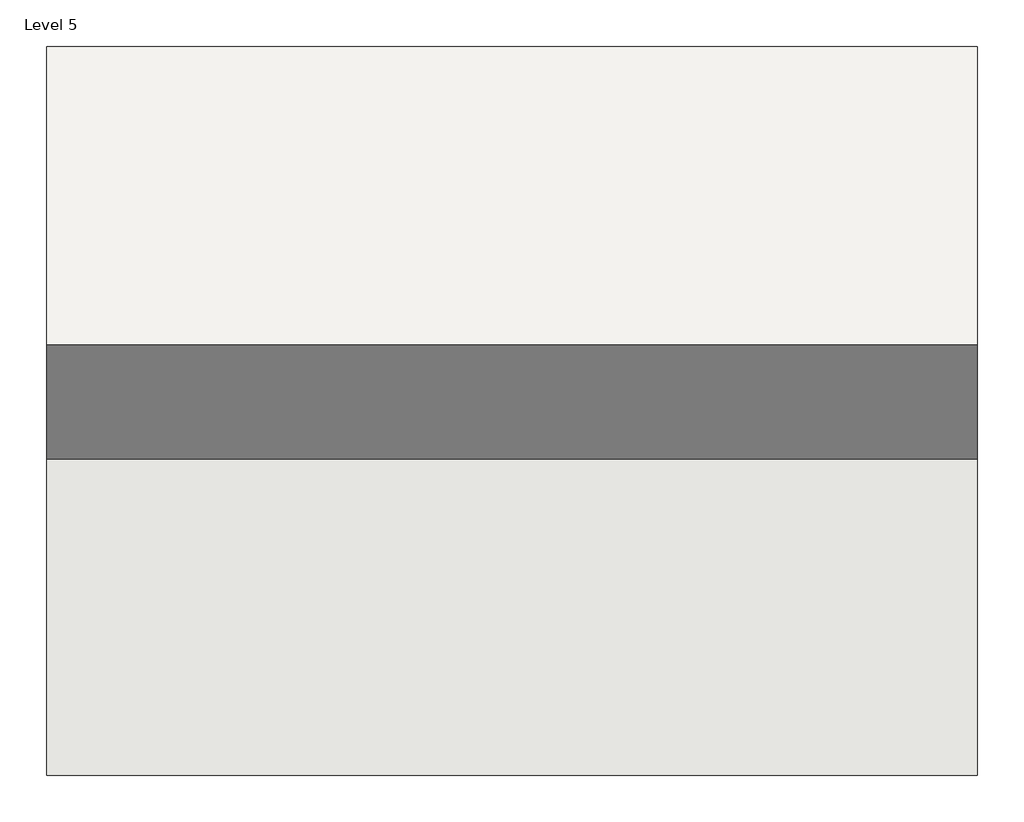
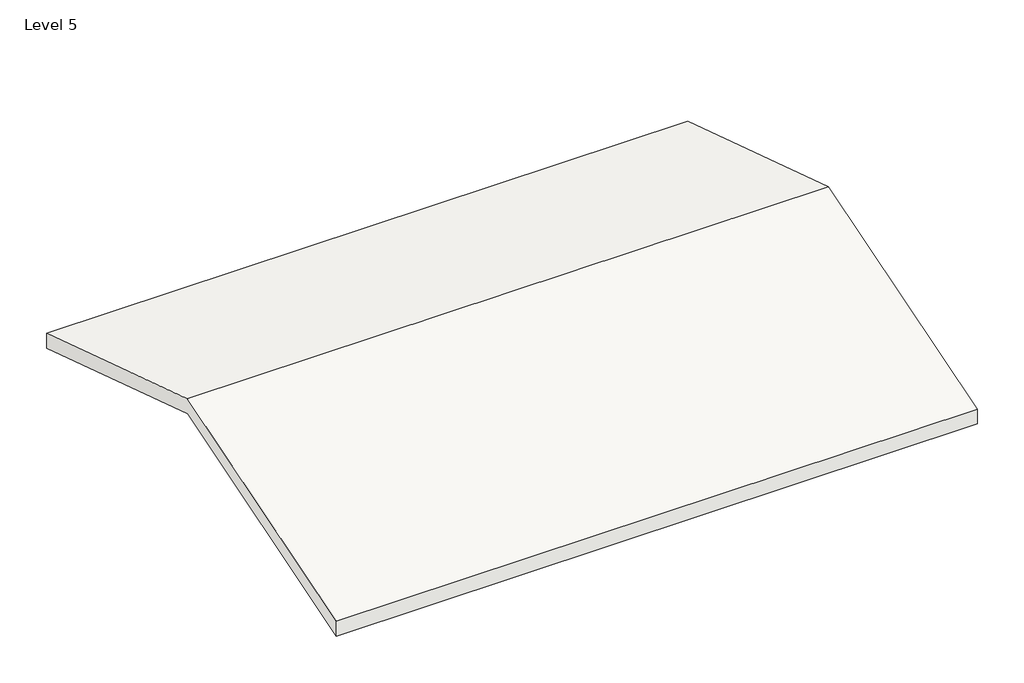
# One storey: 1 roof.
"""IFC4 building model written with IfcOpenShell, lengths in millimetres."""

from ifc_helpers import new_model, si_unit, frame, origin, place, context, project, spatial, polyline, outline, extrude, element, save

model = new_model("IFC4")

# Units and contexts
model_context = context("Model", 3, world=origin())
ifc_project = project(units=[si_unit("LENGTHUNIT", "METRE", prefix="MILLI")], contexts=[model_context])

# Site, building, storey
site = spatial("IfcSite", under=ifc_project)
building = spatial("IfcBuilding", under=site)
storey = spatial("IfcBuildingStorey", under=building, Name="Level 5", Elevation=6400.8)

# Roof
placement = place(None, origin())
element("IfcRoof", 1, ObjectType="Generic - 12\"", at=placement, inside=storey, context=model_context, shape_type="SweptSolid", body=[
    extrude(outline(polyline([(10575.1099631, 6248.4), (10575.1099631, 5928.082294), (5608.4506361, 7532.9678542), (364.3099631, 5929.6731526), (364.3099631, 6248.4), (5610.9803762, 7852.4681208), (10575.1099631, 6248.4)])), frame((-10840.7101751, 0.0, 0.0), z_axis=(1.0, 0.0, 0.0), x_axis=(0.0, 1.0, 0.0)), (0.0, 0.0, 1.0), 13035.2186639),
])

save(model, "model.ifc")

# Revit data of these elements
# Type "Generic - 12\""
#   Assembly Code = "B1020"
# Element 1 (IfcRoof, "Generic - 12\"")
#   built-in parameter 1001710 = 33615
#   Phase Created = New Construction
